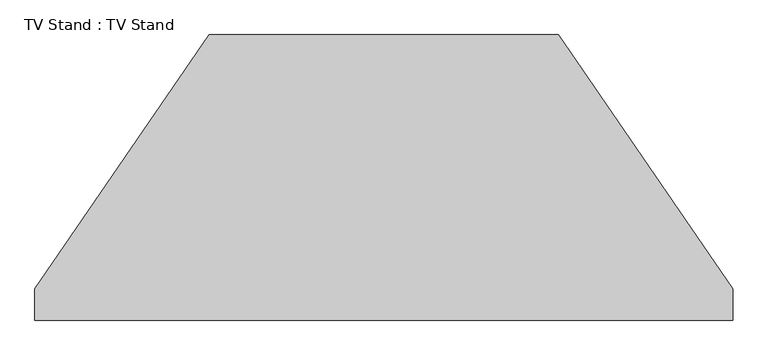
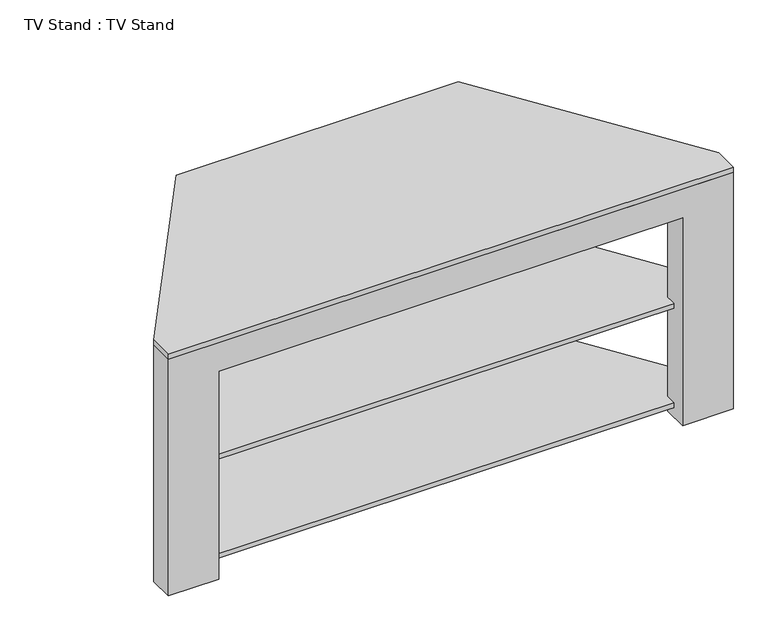
"""IFC4 building model written with IfcOpenShell, lengths in millimetres: furniture geometry, TV Stand : TV Stand."""

from ifc_helpers import new_model, si_unit, point, frame, frame_2d, origin, place, context, project, spatial, polyline, circle_curve, trimmed, segment, composite_curve, outline, extrude, faceted_brep, source, transform, mapped, element, save


def tv_stand_tv_stand_6ce107e5(model_context):
    return source(origin(), model_context, "Body", "SolidModel", [
        extrude(outline(polyline([(425.1724814, -30.0), (633.9880021, -334.3295634), (633.9880021, -427.2), (-383.6119979, -427.2), (-383.6119979, -334.3295634), (-174.7964773, -30.0), (425.1724814, -30.0)])), frame((0.0, 0.0, 20.0), z_axis=(0.0, 0.0, 1.0), x_axis=(1.0, 0.0, 0.0)), (0.0, 0.0, 1.0), 10.0),
        extrude(outline(polyline([(425.1724814, -30.0), (633.9880021, -334.3295634), (633.9880021, -427.2), (-383.6119979, -427.2), (-383.6119979, -334.3295634), (-174.7964773, -30.0), (425.1724814, -30.0)])), frame((0.0, 0.0, 227.65), z_axis=(0.0, 0.0, 1.0), x_axis=(1.0, 0.0, 0.0)), (0.0, 0.0, 1.0), 10.0),
        extrude(outline(polyline([(404.5880021, 0.0), (683.9880021, -407.2), (683.9880021, -457.2), (-433.6119979, -457.2), (-433.6119979, -407.2), (-154.2119979, 0.0), (404.5880021, 0.0)])), frame((0.0, 0.0, 495.3), z_axis=(0.0, 0.0, 1.0), x_axis=(1.0, 0.0, 0.0)), (0.0, 0.0, 1.0), 10.0),
        extrude(outline(polyline([(-50.0, 495.3), (0.0, 495.3), (0.0, 0.0), (-50.0, 0.0), (-50.0, 20.0), (-30.0, 20.0), (-30.0, 30.0), (-50.0, 30.0), (-50.0, 227.65), (-30.0, 227.65), (-30.0, 237.65), (-50.0, 237.65), (-50.0, 495.3)])), frame((-154.2119979, 0.0, 0.0), z_axis=(1.0, 0.0, 0.0), x_axis=(0.0, 1.0, 0.0)), (0.0, 0.0, 1.0), 100.0),
        extrude(outline(polyline([(-50.0, 495.3), (0.0, 495.3), (0.0, 0.0), (-50.0, 0.0), (-50.0, 20.0), (-30.0, 20.0), (-30.0, 30.0), (-50.0, 30.0), (-50.0, 227.65), (-30.0, 227.65), (-30.0, 237.65), (-50.0, 237.65), (-50.0, 495.3)])), frame((304.5880021, 0.0, 0.0), z_axis=(1.0, 0.0, 0.0), x_axis=(0.0, 1.0, 0.0)), (0.0, 0.0, 1.0), 100.0),
        faceted_brep([(-433.6119979, -457.2, 0.0), (-333.6119979, -457.2, 0.0), (-333.6119979, -457.2, 435.3), (583.9880021, -457.2, 435.3), (583.9880021, -457.2, 0.0), (683.9880021, -457.2, 0.0), (683.9880021, -457.2, 495.3), (-433.6119979, -457.2, 495.3), (-433.6119979, -407.2, 0.0), (-433.6119979, -407.2, 495.3), (683.9880021, -407.2, 495.3), (683.9880021, -407.2, 0.0), (583.9880021, -407.2, 0.0), (583.9880021, -407.2, 20.0), (633.9880021, -407.2, 20.0), (633.9880021, -407.2, 30.0), (583.9880021, -407.2, 30.0), (583.9880021, -407.2, 227.65), (633.9880021, -407.2, 227.65), (633.9880021, -407.2, 237.65), (583.9880021, -407.2, 237.65), (583.9880021, -407.2, 435.3), (-333.6119979, -407.2, 435.3), (-333.6119979, -407.2, 237.65), (-383.6119979, -407.2, 237.65), (-383.6119979, -407.2, 227.65), (-333.6119979, -407.2, 227.65), (-333.6119979, -407.2, 30.0), (-383.6119979, -407.2, 30.0), (-383.6119979, -407.2, 20.0), (-333.6119979, -407.2, 20.0), (-333.6119979, -407.2, 0.0), (-333.6119979, -427.2, 20.0), (-333.6119979, -427.2, 30.0), (-333.6119979, -427.2, 227.65), (-333.6119979, -427.2, 237.65), (583.9880021, -427.2, 237.65), (583.9880021, -427.2, 227.65), (583.9880021, -427.2, 30.0), (583.9880021, -427.2, 20.0), (633.9880021, -427.2, 237.65), (-383.6119979, -427.2, 237.65), (-383.6119979, -427.2, 227.65), (633.9880021, -427.2, 227.65), (633.9880021, -427.2, 30.0), (-383.6119979, -427.2, 30.0), (-383.6119979, -427.2, 20.0), (633.9880021, -427.2, 20.0)], [[[0, 1, 2, 3, 4, 5, 6, 7]], [[8, 9, 10, 11, 12, 13, 14, 15, 16, 17, 18, 19, 20, 21, 22, 23, 24, 25, 26, 27, 28, 29, 30, 31]], [[1, 0, 8, 31]], [[2, 1, 31, 30, 32, 33, 27, 26, 34, 35, 23, 22]], [[3, 2, 22, 21]], [[4, 3, 21, 20, 36, 37, 17, 16, 38, 39, 13, 12]], [[5, 4, 12, 11]], [[6, 5, 11, 10]], [[7, 6, 10, 9]], [[0, 7, 9, 8]], [[19, 40, 36, 20]], [[35, 41, 24, 23]], [[25, 42, 34, 26]], [[37, 43, 18, 17]], [[41, 42, 25, 24]], [[42, 41, 35, 34]], [[40, 43, 37, 36]], [[43, 40, 19, 18]], [[15, 44, 38, 16]], [[33, 45, 28, 27]], [[29, 46, 32, 30]], [[39, 47, 14, 13]], [[45, 46, 29, 28]], [[46, 45, 33, 32]], [[44, 47, 39, 38]], [[47, 44, 15, 14]]]),
        extrude(outline(polyline([(0.0, 304.5880021), (495.3, 304.5880021), (495.3, -54.2119979), (0.0, -54.2119979), (0.0, 304.5880021)]), holes=[composite_curve([segment(polyline([(242.65, 145.1700818), (242.65, 105.2059224)]), True, "CONTINUOUS"), segment(trimmed(circle_curve(frame_2d((255.15, 105.2059224)), 12.5), [point((242.65, 105.2059224))], [point((267.65, 105.2059224))], True, "CARTESIAN"), True, "CONTINUOUS"), segment(polyline([(267.65, 105.2059224), (267.65, 145.1700818)]), True, "CONTINUOUS"), segment(trimmed(circle_curve(frame_2d((255.15, 145.1700818)), 12.5), [point((267.65, 145.1700818))], [point((242.65, 145.1700818))], True, "CARTESIAN"), True, "CONTINUOUS")], self_intersect=False), composite_curve([segment(polyline([(35.0, 145.1880021), (35.0, 105.2059224)]), True, "CONTINUOUS"), segment(trimmed(circle_curve(frame_2d((47.5, 105.2059224)), 12.5), [point((35.0, 105.2059224))], [point((60.0, 105.2059224))], True, "CARTESIAN"), True, "CONTINUOUS"), segment(polyline([(60.0, 105.2059224), (60.0, 145.1880021)]), True, "CONTINUOUS"), segment(trimmed(circle_curve(frame_2d((47.5, 145.1880021)), 12.5), [point((60.0, 145.1880021))], [point((35.0, 145.1880021))], True, "CARTESIAN"), True, "CONTINUOUS")], self_intersect=False)]), frame((0.0, -30.0, 0.0), z_axis=(0.0, 1.0, 0.0), x_axis=(0.0, 0.0, 1.0)), (0.0, 0.0, 1.0), 10.0),
    ])


if __name__ == "__main__":
    model = new_model("IFC4")
    model_context = context("Model", 3, world=origin())
    ifc_project = project(units=[si_unit("LENGTHUNIT", "METRE", prefix="MILLI")], contexts=[model_context])
    site = spatial("IfcSite", under=ifc_project)
    building = spatial("IfcBuilding", under=site)
    placement = place(None, origin())
    tv_stand_tv_stand_shape = tv_stand_tv_stand_6ce107e5(model_context)
    element("IfcFurniture", 1, ObjectType="TV Stand : TV Stand", at=placement, inside=building, context=model_context, shape_type="MappedRepresentation", body=[
        mapped(tv_stand_tv_stand_shape, transform((0.0, 0.0, 0.0), x_axis=(1.0, 0.0, 0.0), y_axis=(0.0, 1.0, 0.0), z_axis=(0.0, 0.0, 1.0))),
    ])
    save(model, "model.ifc")

# Revit data of these elements
# Type "TV Stand : TV Stand"
#   Depth = 1' - 6"
#   Width = 3' - 8"
#   Height = 1' - 7 1/2"
#   Finish = Melamine - Gray
# Element 1 (IfcFurniture, "TV Stand : TV Stand")
#   Materials on its faces: "Melamine - Gray", "Glass - Shelves"
# Materials
#   "Melamine - Gray": class "Wood", colour RGB 49 49 49, transparency 0
#   "Glass - Shelves": class "Glass", colour RGB 167 167 167, transparency 0.9
